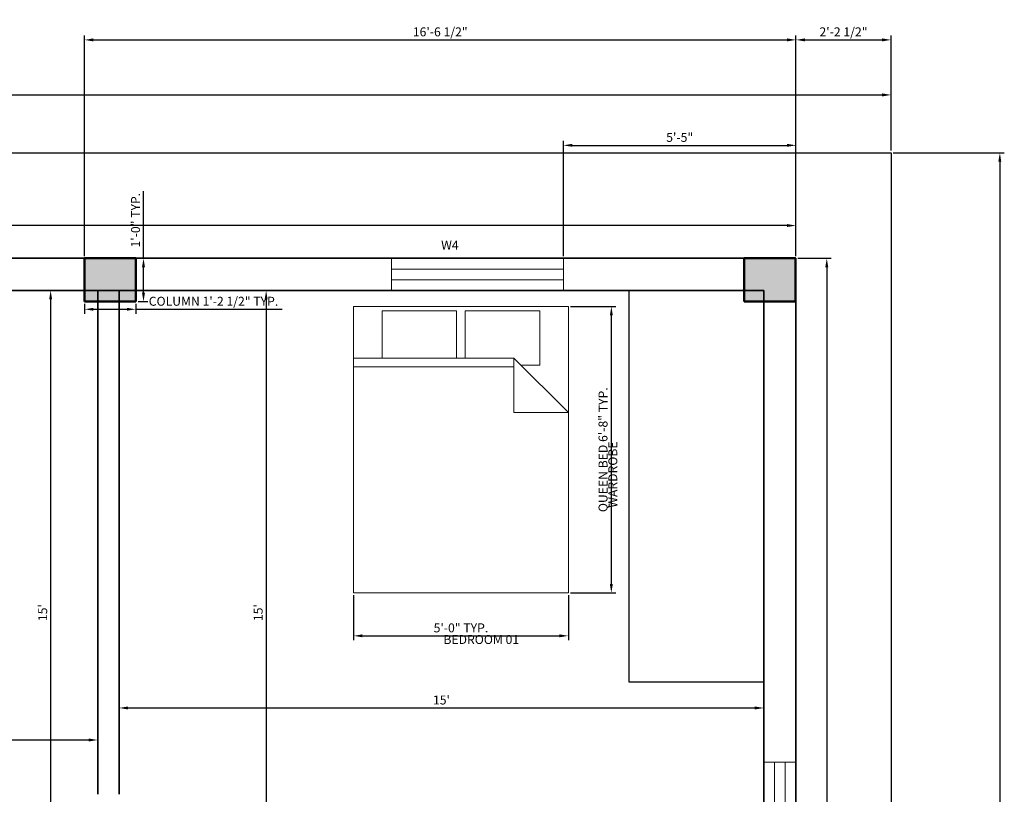
# Model space of a CAD drawing. Units: inches. Extents: x 2470 to 6338, y 1562 to 4199.
# Tile 4 of 5: x 2803 to 3078, y 1985 to 2201. Entities that reach past the tile are written whole.
import ezdxf

# ---------------------------------------------------------------- set-up
doc = ezdxf.new("R2010")
doc.units = ezdxf.units.IN
for name, color, linetype, lineweight in [('A-ANNO-DIMS', 2, 'Continuous', 18), ('A-ANNO-TEXT', 7, 'Continuous', 18), ('A-AREA-IDEN', 7, 'Continuous', 25), ('A-COLS', 1, 'Continuous', 50), ('A-FURN', 8, 'Continuous', 18), ('A-FURN-FIXD', 8, 'Continuous', 25), ('A-GLAZ', 4, 'Continuous', 18), ('A-WALL', 7, 'Continuous', 35), ('C-PROP', 3, 'Continuous', 25)]:
    doc.layers.add(name, color=color, linetype=linetype, lineweight=lineweight)
doc.styles.get("Standard").update_dxf_attribs({"font": 'arial.ttf'})
doc.dimstyles.new('ISO-25', dxfattribs={"dimtxt": 2.5, "dimasz": 2.5, "dimexe": 1.25, "dimexo": 0.625, "dimtad": 1, "dimdec": 1, "dimlunit": 3, "dimtxsty": 'Standard', "dimcen": 2.5, "dimadec": 0, "dimazin": 0, "dimtfac": 1, "dimtdec": 1, "dimtmove": 0, "dimatfit": 3, "dimfxl": 1, "dimarcsym": 0})

# ---------------------------------------------------------------- blocks, each defined once
blk = doc.blocks.new('Bed - Queen')
for p, q in [((0, -80.00003), (0, 0)), ((0, 0), (59.99999, 0)), ((59.99999, 0), (59.99999, -80.00003)), ((7.99999, -1.2), (28.79998, -1.2)), ((7.99999, -14.4), (7.99999, -1.2)), ((28.79998, -1.2), (28.79998, -14.4)), ((31.19999, -1.2), (51.99999, -1.2)), ((31.19999, -14.4), (31.19999, -1.2)), ((51.99999, -1.2), (51.99999, -16.4)), ((0, -14.4), (44.8, -14.4)), ((59.99999, -29.6), (44.8, -14.4)), ((44.8, -14.4), (44.8, -29.6)), ((51.99999, -16.4), (46.79936, -16.4)), ((44.8, -16.8), (0, -16.8)), ((44.8, -29.6), (59.99999, -29.6)), ((59.99999, -80.00003), (0, -80.00003))]:
    blk.add_line(p, q)
blk = doc.blocks.new('*D8')
at = {"layer": 'A-ANNO-DIMS', "color": 0, "lineweight": -2, "transparency": 16777216}
for p, q in [((2530.72, 2164.62), (2530.72, 2181.42)), ((3046.72, 2164.62), (3046.72, 2181.42)), ((2533.22, 2180.17), (3044.22, 2180.17))]:
    blk.add_line(p, q, dxfattribs=at)
at = {"layer": 'A-ANNO-DIMS', "color": 0, "lineweight": 100, "transparency": 16777216}
for points in [[(2533.22, 2180.59), (2533.22, 2179.75), (2530.72, 2180.17)], [(3044.22, 2180.59), (3044.22, 2179.75), (3046.72, 2180.17)]]:
    blk.add_solid(points, dxfattribs=at)
at = {"layer": 'Defpoints', "color": 0, "lineweight": 100, "transparency": 16777216}
for p in [(3046.72, 2180.17), (2530.72, 2163.99), (3046.72, 2163.99)]:
    blk.add_point(p, dxfattribs=at)
at = {"layer": 'A-ANNO-DIMS', "color": 0, "transparency": 16777216, "insert": (2788.72, 2182.07), "char_height": 2.5, "attachment_point": 5}
blk.add_mtext("43'", dxfattribs=at)
blk = doc.blocks.new('*D9')
at = {"layer": 'A-ANNO-DIMS', "color": 0, "lineweight": -2, "transparency": 16777216}
for p, q in [((3047.35, 2163.99), (3078.35, 2163.99)), ((3077.1, 2161.49), (3077.1, 1597.49)), ((3047.35, 1594.99), (3078.35, 1594.99))]:
    blk.add_line(p, q, dxfattribs=at)
at = {"layer": 'A-ANNO-DIMS', "color": 0, "lineweight": 100, "transparency": 16777216}
for points in [[(3076.68, 2161.49), (3077.51, 2161.49), (3077.1, 2163.99)], [(3076.68, 1597.49), (3077.51, 1597.49), (3077.1, 1594.99)]]:
    blk.add_solid(points, dxfattribs=at)
at = {"layer": 'Defpoints', "color": 0, "lineweight": 100, "transparency": 16777216}
for p in [(3046.72, 2163.99), (3046.72, 1594.99), (3077.1, 1594.99)]:
    blk.add_point(p, dxfattribs=at)
at = {"layer": 'A-ANNO-DIMS', "color": 0, "transparency": 16777216, "insert": (3075.2, 1879.49), "char_height": 2.5, "attachment_point": 5, "rotation": 90}
blk.add_mtext('47\'-5"', dxfattribs=at)
blk = doc.blocks.new('*D11')
at = {"layer": 'A-ANNO-DIMS', "color": 0, "lineweight": -2, "transparency": 16777216}
for p, q in [((2576.17, 2135.16), (2576.17, 2144.92)), ((3020.17, 2135.16), (3020.17, 2144.92)), ((3017.67, 2143.67), (2578.67, 2143.67))]:
    blk.add_line(p, q, dxfattribs=at)
at = {"layer": 'A-ANNO-DIMS', "color": 0, "lineweight": 100, "transparency": 16777216}
for points in [[(2578.67, 2144.09), (2578.67, 2143.26), (2576.17, 2143.67)], [(3017.67, 2144.09), (3017.67, 2143.26), (3020.17, 2143.67)]]:
    blk.add_solid(points, dxfattribs=at)
at = {"layer": 'Defpoints', "color": 0, "lineweight": 100, "transparency": 16777216}
for p in [(2576.17, 2143.67), (2576.17, 2134.53), (3020.17, 2134.53)]:
    blk.add_point(p, dxfattribs=at)
at = {"layer": 'A-ANNO-DIMS', "color": 0, "transparency": 16777216, "insert": (2798.17, 2145.58), "char_height": 2.5, "attachment_point": 5}
blk.add_mtext("37'", dxfattribs=at)
blk = doc.blocks.new('*D12')
at = {"layer": 'A-ANNO-DIMS', "color": 0, "lineweight": -2, "transparency": 16777216}
for p, q in [((3020.65, 2134.53), (3030.02, 2134.53)), ((3028.77, 2132.03), (3028.77, 1753.03)), ((3020.65, 1750.53), (3030.02, 1750.53))]:
    blk.add_line(p, q, dxfattribs=at)
at = {"layer": 'A-ANNO-DIMS', "color": 0, "lineweight": 100, "transparency": 16777216}
for points in [[(3028.36, 2132.03), (3029.19, 2132.03), (3028.77, 2134.53)], [(3028.36, 1753.03), (3029.19, 1753.03), (3028.77, 1750.53)]]:
    blk.add_solid(points, dxfattribs=at)
at = {"layer": 'Defpoints', "color": 0, "lineweight": 100, "transparency": 16777216}
for p in [(3020.03, 2134.53), (3020.03, 1750.53), (3028.77, 1750.53)]:
    blk.add_point(p, dxfattribs=at)
at = {"layer": 'A-ANNO-DIMS', "color": 0, "transparency": 16777216, "insert": (3026.87, 1942.53), "char_height": 2.5, "attachment_point": 5, "rotation": 90}
blk.add_mtext("32'", dxfattribs=at)
blk = doc.blocks.new('*D27')
at = {"layer": 'A-ANNO-DIMS', "color": 0, "lineweight": -2, "transparency": 16777216}
for p, q in [((2711.17, 2058.91), (2711.17, 1998.69)), ((2825.17, 2058.91), (2825.17, 1998.69)), ((2713.67, 1999.94), (2822.67, 1999.94))]:
    blk.add_line(p, q, dxfattribs=at)
at = {"layer": 'A-ANNO-DIMS', "color": 0, "lineweight": 100, "transparency": 16777216}
for points in [[(2713.67, 2000.36), (2713.67, 1999.53), (2711.17, 1999.94)], [(2822.67, 2000.36), (2822.67, 1999.53), (2825.17, 1999.94)]]:
    blk.add_solid(points, dxfattribs=at)
at = {"layer": 'Defpoints', "color": 0, "lineweight": 100, "transparency": 16777216}
for p in [(2711.17, 2059.53), (2825.17, 2059.53), (2825.17, 1999.94)]:
    blk.add_point(p, dxfattribs=at)
at = {"layer": 'A-ANNO-DIMS', "color": 0, "transparency": 16777216, "insert": (2768.17, 2001.84), "char_height": 2.5, "attachment_point": 5}
blk.add_mtext('9\'-6"', dxfattribs=at)
blk = doc.blocks.new('*D28')
at = {"layer": 'A-ANNO-DIMS', "color": 0, "lineweight": -2, "transparency": 16777216}
for p, q in [((2808.15, 2125.53), (2813.28, 2125.53)), ((2812.03, 2123.03), (2812.03, 1948.03)), ((2808.15, 1945.53), (2813.28, 1945.53))]:
    blk.add_line(p, q, dxfattribs=at)
at = {"layer": 'A-ANNO-DIMS', "color": 0, "lineweight": 100, "transparency": 16777216}
for points in [[(2811.62, 2123.03), (2812.45, 2123.03), (2812.03, 2125.53)], [(2811.62, 1948.03), (2812.45, 1948.03), (2812.03, 1945.53)]]:
    blk.add_solid(points, dxfattribs=at)
at = {"layer": 'Defpoints', "color": 0, "lineweight": 100, "transparency": 16777216}
for p in [(2807.53, 2125.53), (2807.53, 1945.53), (2812.03, 1945.53)]:
    blk.add_point(p, dxfattribs=at)
at = {"layer": 'A-ANNO-DIMS', "color": 0, "transparency": 16777216, "insert": (2810.13, 2035.53), "char_height": 2.5, "attachment_point": 5, "rotation": 90}
blk.add_mtext("15'", dxfattribs=at)
blk = doc.blocks.new('*D29')
at = {"layer": 'A-ANNO-DIMS', "color": 0, "lineweight": -2, "transparency": 16777216}
for p, q in [((2831.17, 2010.54), (2831.17, 2007.64)), ((3011.17, 2010.54), (3011.17, 2007.64)), ((2833.67, 2008.89), (3008.67, 2008.89))]:
    blk.add_line(p, q, dxfattribs=at)
at = {"layer": 'A-ANNO-DIMS', "color": 0, "lineweight": 100, "transparency": 16777216}
for points in [[(2833.67, 2009.31), (2833.67, 2008.47), (2831.17, 2008.89)], [(3008.67, 2009.31), (3008.67, 2008.47), (3011.17, 2008.89)]]:
    blk.add_solid(points, dxfattribs=at)
at = {"layer": 'Defpoints', "color": 0, "lineweight": 100, "transparency": 16777216}
for p in [(2831.17, 2011.17), (3011.17, 2011.17), (3011.17, 2008.89)]:
    blk.add_point(p, dxfattribs=at)
at = {"layer": 'A-ANNO-DIMS', "color": 0, "transparency": 16777216, "insert": (2921.17, 2010.79), "char_height": 2.5, "attachment_point": 5}
blk.add_mtext("15'", dxfattribs=at)
blk = doc.blocks.new('*D30')
at = {"layer": 'A-ANNO-DIMS', "color": 0, "lineweight": -2, "transparency": 16777216}
for p, q in [((2859.5, 2125.53), (2873.46, 2125.53)), ((2872.21, 2123.03), (2872.21, 1948.03)), ((2867.05, 1945.53), (2873.46, 1945.53))]:
    blk.add_line(p, q, dxfattribs=at)
at = {"layer": 'A-ANNO-DIMS', "color": 0, "lineweight": 100, "transparency": 16777216}
for points in [[(2871.79, 2123.03), (2872.62, 2123.03), (2872.21, 2125.53)], [(2871.79, 1948.03), (2872.62, 1948.03), (2872.21, 1945.53)]]:
    blk.add_solid(points, dxfattribs=at)
at = {"layer": 'Defpoints', "color": 0, "lineweight": 100, "transparency": 16777216}
for p in [(2858.88, 2125.53), (2866.42, 1945.53), (2872.21, 1945.53)]:
    blk.add_point(p, dxfattribs=at)
at = {"layer": 'A-ANNO-DIMS', "color": 0, "transparency": 16777216, "insert": (2870.31, 2035.53), "char_height": 2.5, "attachment_point": 5, "rotation": 90}
blk.add_mtext("15'", dxfattribs=at)
blk = doc.blocks.new('WIN-48IN')
for p, q in [((0, 9), (48, 9)), ((0, 0), (0, 9)), ((48, 9), (48, 0)), ((0, 6), (48, 6)), ((48, 3), (0, 3)), ((48, 0), (0, 0))]:
    blk.add_line(p, q)
blk = doc.blocks.new('COL-RECT-LARGE')
h = blk.add_hatch(color=256)
h.dxf.hatch_style = 1
h.paths.add_polyline_path([(14.33, 12.11), (10, 12.11), (0, 12.11), (0, 0), (10, 0), (14.33, 0)])
for p, q in [((10, 12.11), (0, 12.11)), ((0, 12.11), (0, 0)), ((10, 12.11), (14.33, 12.11)), ((14.33, 12.11), (14.33, 0)), ((10, 0), (0, 0)), ((14.33, 0), (10, 0))]:
    blk.add_line(p, q)
blk = doc.blocks.new('*D40')
at = {"layer": 'A-ANNO-DIMS', "color": 0, "lineweight": -2, "transparency": 16777216}
for p, q in [((2821.49, 2121.8), (2821.49, 2119.03)), ((2823.99, 2120.28), (2833.31, 2120.28)), ((2835.81, 2121.8), (2835.81, 2119.03)), ((2835.81, 2120.28), (2876.7, 2120.28))]:
    blk.add_line(p, q, dxfattribs=at)
at = {"layer": 'A-ANNO-DIMS', "color": 0, "lineweight": 100, "transparency": 16777216}
for points in [[(2823.99, 2120.69), (2823.99, 2119.86), (2821.49, 2120.28)], [(2833.31, 2120.69), (2833.31, 2119.86), (2835.81, 2120.28)]]:
    blk.add_solid(points, dxfattribs=at)
at = {"layer": 'Defpoints', "color": 0, "lineweight": 100, "transparency": 16777216}
for p in [(2821.49, 2122.42), (2835.81, 2122.42), (2835.81, 2120.28)]:
    blk.add_point(p, dxfattribs=at)
at = {"layer": 'A-ANNO-DIMS', "color": 0, "transparency": 16777216, "insert": (2857.51, 2122.19), "char_height": 2.5, "attachment_point": 5}
blk.add_mtext('COLUMN 1\'-2 1/2" TYP.', dxfattribs=at)
blk = doc.blocks.new('*D41')
at = {"layer": 'A-ANNO-DIMS', "color": 0, "lineweight": -2, "transparency": 16777216}
for p, q in [((2837.96, 2134.53), (2837.96, 2153.29)), ((2836.44, 2134.53), (2839.21, 2134.53)), ((2837.96, 2124.92), (2837.96, 2132.03)), ((2836.44, 2122.42), (2839.21, 2122.42))]:
    blk.add_line(p, q, dxfattribs=at)
at = {"layer": 'A-ANNO-DIMS', "color": 0, "lineweight": 100, "transparency": 16777216}
for points in [[(2837.54, 2132.03), (2838.38, 2132.03), (2837.96, 2134.53)], [(2837.54, 2124.92), (2838.38, 2124.92), (2837.96, 2122.42)]]:
    blk.add_solid(points, dxfattribs=at)
at = {"layer": 'Defpoints', "color": 0, "lineweight": 100, "transparency": 16777216}
for p in [(2835.81, 2134.53), (2837.96, 2134.53), (2835.81, 2122.42)]:
    blk.add_point(p, dxfattribs=at)
at = {"layer": 'A-ANNO-DIMS', "color": 0, "transparency": 16777216, "insert": (2836.06, 2145.16), "char_height": 2.5, "attachment_point": 5, "rotation": 90}
blk.add_mtext('1\'-0" TYP.', dxfattribs=at)
blk = doc.blocks.new('*D46')
at = {"layer": 'A-ANNO-DIMS', "color": 0, "lineweight": -2, "transparency": 16777216}
for p, q in [((2957.23, 2121.04), (2969.86, 2121.04)), ((2968.61, 2043.54), (2968.61, 2118.54)), ((2957.23, 2041.04), (2969.86, 2041.04))]:
    blk.add_line(p, q, dxfattribs=at)
at = {"layer": 'A-ANNO-DIMS', "color": 0, "lineweight": 100, "transparency": 16777216}
for points in [[(2968.19, 2118.54), (2969.03, 2118.54), (2968.61, 2121.04)], [(2968.19, 2043.54), (2969.03, 2043.54), (2968.61, 2041.04)]]:
    blk.add_solid(points, dxfattribs=at)
at = {"layer": 'Defpoints', "color": 0, "lineweight": 100, "transparency": 16777216}
for p in [(2956.61, 2121.04), (2968.61, 2121.04), (2956.61, 2041.04)]:
    blk.add_point(p, dxfattribs=at)
at = {"layer": 'A-ANNO-DIMS', "color": 0, "transparency": 16777216, "insert": (2966.61, 2081.04), "char_height": 2.5, "attachment_point": 5, "rotation": 90}
blk.add_mtext('QUEEN BED 6\'-8" TYP.', dxfattribs=at)
blk = doc.blocks.new('*D47')
at = {"layer": 'A-ANNO-DIMS', "color": 0, "lineweight": -2, "transparency": 16777216}
for p, q in [((2896.61, 2040.42), (2896.61, 2027.79)), ((2956.61, 2040.42), (2956.61, 2027.79)), ((2899.11, 2029.04), (2954.11, 2029.04))]:
    blk.add_line(p, q, dxfattribs=at)
at = {"layer": 'A-ANNO-DIMS', "color": 0, "lineweight": 100, "transparency": 16777216}
for points in [[(2899.11, 2029.46), (2899.11, 2028.63), (2896.61, 2029.04)], [(2954.11, 2029.46), (2954.11, 2028.63), (2956.61, 2029.04)]]:
    blk.add_solid(points, dxfattribs=at)
at = {"layer": 'Defpoints', "color": 0, "lineweight": 100, "transparency": 16777216}
for p in [(2896.61, 2041.04), (2956.61, 2041.04), (2956.61, 2029.04)]:
    blk.add_point(p, dxfattribs=at)
at = {"layer": 'A-ANNO-DIMS', "color": 0, "transparency": 16777216, "insert": (2926.61, 2030.94), "char_height": 2.5, "attachment_point": 5}
blk.add_mtext('5\'-0" TYP.', dxfattribs=at)
blk = doc.blocks.new('*D61')
at = {"layer": 'A-ANNO-DIMS', "color": 0, "lineweight": -2, "transparency": 16777216}
for p, q in [((2821.49, 2135.16), (2821.49, 2196.79)), ((2823.99, 2195.54), (3017.67, 2195.54)), ((3020.17, 2135.16), (3020.17, 2196.79))]:
    blk.add_line(p, q, dxfattribs=at)
at = {"layer": 'A-ANNO-DIMS', "color": 0, "lineweight": 100, "transparency": 16777216}
for points in [[(2823.99, 2195.96), (2823.99, 2195.12), (2821.49, 2195.54)], [(3017.67, 2195.96), (3017.67, 2195.12), (3020.17, 2195.54)]]:
    blk.add_solid(points, dxfattribs=at)
at = {"layer": 'Defpoints', "color": 0, "lineweight": 100, "transparency": 16777216}
for p in [(3020.17, 2195.54), (2821.49, 2134.53), (3020.17, 2134.53)]:
    blk.add_point(p, dxfattribs=at)
at = {"layer": 'A-ANNO-DIMS', "color": 0, "transparency": 16777216, "insert": (2920.83, 2197.46), "char_height": 2.5, "attachment_point": 5}
blk.add_mtext('16\'-6 1/2"', dxfattribs=at)
blk = doc.blocks.new('*D66')
at = {"layer": 'A-ANNO-DIMS', "color": 0, "lineweight": -2, "transparency": 16777216}
for p, q in [((3020.17, 2135.16), (3020.17, 2196.79)), ((3022.67, 2195.54), (3044.22, 2195.54)), ((3046.72, 2164.62), (3046.72, 2196.79))]:
    blk.add_line(p, q, dxfattribs=at)
at = {"layer": 'A-ANNO-DIMS', "color": 0, "lineweight": 100, "transparency": 16777216}
for points in [[(3022.67, 2195.96), (3022.67, 2195.12), (3020.17, 2195.54)], [(3044.22, 2195.96), (3044.22, 2195.12), (3046.72, 2195.54)]]:
    blk.add_solid(points, dxfattribs=at)
at = {"layer": 'Defpoints', "color": 0, "lineweight": 100, "transparency": 16777216}
for p in [(3046.72, 2195.54), (3046.72, 2163.99), (3020.17, 2134.53)]:
    blk.add_point(p, dxfattribs=at)
at = {"layer": 'A-ANNO-DIMS', "color": 0, "transparency": 16777216, "insert": (3033.44, 2197.46), "char_height": 2.5, "attachment_point": 5}
blk.add_mtext('2\'-2 1/2"', dxfattribs=at)
blk = doc.blocks.new('*D72')
at = {"layer": 'A-ANNO-DIMS', "color": 0, "lineweight": -2, "transparency": 16777216}
for p, q in [((2955.23, 2135.16), (2955.23, 2167.33)), ((3020.17, 2135.16), (3020.17, 2167.33)), ((2957.73, 2166.08), (3017.67, 2166.08))]:
    blk.add_line(p, q, dxfattribs=at)
at = {"layer": 'A-ANNO-DIMS', "color": 0, "lineweight": 100, "transparency": 16777216}
for points in [[(2957.73, 2166.5), (2957.73, 2165.67), (2955.23, 2166.08)], [(3017.67, 2166.5), (3017.67, 2165.67), (3020.17, 2166.08)]]:
    blk.add_solid(points, dxfattribs=at)
at = {"layer": 'Defpoints', "color": 0, "lineweight": 100, "transparency": 16777216}
for p in [(3020.17, 2166.08), (2955.23, 2134.53), (3020.17, 2134.53)]:
    blk.add_point(p, dxfattribs=at)
at = {"layer": 'A-ANNO-DIMS', "color": 0, "transparency": 16777216, "insert": (2987.7, 2167.98), "char_height": 2.5, "attachment_point": 5}
blk.add_mtext('5\'-5"', dxfattribs=at)

msp = doc.modelspace()

# ---------------------------------------------------------------- linework, layer by layer
at = {"layer": 'A-FURN-FIXD'}
for p, q in [((2973.48, 2125.53), (2973.48, 2016.18)), ((2973.48, 2016.18), (3011.17, 2016.18))]:
    msp.add_line(p, q, dxfattribs=at)
at = {"layer": 'A-WALL'}
for p, q in [((2576.17, 2134.53), (3020.17, 2134.53)), ((3020.17, 2134.53), (3020.17, 1750.53)), ((2585.17, 2125.53), (3011.17, 2125.53)), ((2825.17, 2125.53), (2825.17, 1984.76)), ((2831.17, 2125.53), (2831.17, 1984.76)), ((3011.17, 2125.53), (3011.17, 1852.53))]:
    msp.add_line(p, q, dxfattribs=at)
at = {"layer": 'C-PROP'}
for p, q in [((2530.72, 2163.99), (3046.72, 2163.99)), ((3046.72, 2163.99), (3046.72, 1594.99))]:
    msp.add_line(p, q, dxfattribs=at)

# ---------------------------------------------------------------- block references
at = {"layer": 'A-COLS'}
for p in [(2821.49, 2122.42), (3005.7, 2122.42)]:
    msp.add_blockref('COL-RECT-LARGE', p, dxfattribs=at)
at = {"layer": 'A-FURN'}
msp.add_blockref('Bed - Queen', (2896.61, 2121.04), dxfattribs=at)
at = {"layer": 'A-GLAZ'}
msp.add_blockref('WIN-48IN', (2907.23, 2125.53), dxfattribs=at)
at = {"layer": 'A-GLAZ', "rotation": 89.9999999999996}
msp.add_blockref('WIN-48IN', (3020.17, 1945.73), dxfattribs=at)

# ---------------------------------------------------------------- texts
at = {"layer": 'A-ANNO-TEXT', "insert": (2921.08, 2139.44), "char_height": 2.5, "attachment_point": 1}
msp.add_mtext_dynamic_manual_height_columns('W4', width=14.944, gutter_width=12.5, heights=[0], dxfattribs=at)
at = {"layer": 'A-ANNO-TEXT', "insert": (2967.77, 2064.83), "char_height": 2.5, "attachment_point": 1, "rotation": 90}
msp.add_mtext_dynamic_manual_height_columns('WARDROBE', width=31.0449, gutter_width=12.5, heights=[0], dxfattribs=at)
at = {"layer": 'A-AREA-IDEN', "insert": (2921.71, 2029.26), "char_height": 2.5, "attachment_point": 1}
msp.add_mtext_dynamic_manual_height_columns('BEDROOM 01', width=53.323, gutter_width=12.5, heights=[0], dxfattribs=at)

# ---------------------------------------------------------------- dimensions: what is measured, and where the dimension line sits
at = {"layer": 'A-ANNO-DIMS'}
for base, p1, p2, override, picture, middle in [((3020.17, 2195.54), (2821.49, 2134.53), (3020.17, 2134.53), {"dimdec": 1, "dimlfac": 1, "dimrnd": 0, "dimzin": 1, "dimdsep": 46, "dimlunit": 4, "dimfrac": 2}, '*D61', (2920.83, 2197.46)), ((3046.7223, 2195.5407), (3020.1674, 2134.5342), (3046.7223, 2163.9907), {"dimdec": 1, "dimlfac": 1, "dimrnd": 0, "dimzin": 1, "dimdsep": 46, "dimlunit": 4, "dimfrac": 2}, '*D66', (3033.4449, 2197.4584)), ((3046.72, 2180.17), (2530.72, 2163.99), (3046.72, 2163.99), {"dimclrd": 0, "dimclre": 0, "dimclrt": 0}, '*D8', (2788.72, 2182.07)), ((3020.17, 2166.08), (2955.23, 2134.53), (3020.17, 2134.53), {"dimdec": 1, "dimlfac": 1, "dimrnd": 0, "dimzin": 1, "dimdsep": 46, "dimlunit": 4, "dimfrac": 2}, '*D72', (2987.7, 2167.98)), ((2576.17, 2143.67), (3020.17, 2134.53), (2576.17, 2134.53), {"dimclrd": 0, "dimclre": 0, "dimclrt": 0}, '*D11', (2798.17, 2145.58)), ((2825.17, 1999.94), (2711.17, 2059.53), (2825.17, 2059.53), {"dimclrd": 0, "dimclre": 0, "dimclrt": 0}, '*D27', (2768.17, 2001.84)), ((3011.17, 2008.89), (2831.17, 2011.17), (3011.17, 2011.17), {"dimclrd": 0, "dimclre": 0, "dimclrt": 0}, '*D29', (2921.17, 2010.79))]:
    dim = msp.add_linear_dim(base=base, p1=p1, p2=p2, dimstyle='ISO-25', override=override, dxfattribs=at)
    dim.commit()
    dim.dimension.update_dxf_attribs({"geometry": picture, "text_midpoint": middle})
for base, p1, p2, picture, middle in [((3077.1, 1594.99), (3046.72, 2163.99), (3046.72, 1594.99), '*D9', (3075.2, 1879.49)), ((3028.77, 1750.53), (3020.03, 2134.53), (3020.03, 1750.53), '*D12', (3026.87, 1942.53)), ((2812.03, 1945.53), (2807.53, 2125.53), (2807.53, 1945.53), '*D28', (2810.13, 2035.53)), ((2872.21, 1945.53), (2858.88, 2125.53), (2866.42, 1945.53), '*D30', (2870.31, 2035.53))]:
    dim = msp.add_linear_dim(base=base, p1=p1, p2=p2, angle=90, dimstyle='ISO-25', override={"dimclrd": 0, "dimclre": 0, "dimclrt": 0}, dxfattribs=at)
    dim.commit()
    dim.dimension.update_dxf_attribs({"geometry": picture, "text_midpoint": middle})
for base, p1, p2, text, picture, middle in [((2837.96, 2134.53), (2835.81, 2122.42), (2835.81, 2134.53), '<> TYP.', '*D41', (2836.06, 2145.16)), ((2968.61, 2121.04), (2956.61, 2041.04), (2956.61, 2121.04), 'QUEEN BED <> TYP.', '*D46', (2966.61, 2081.04))]:
    dim = msp.add_linear_dim(base=base, p1=p1, p2=p2, angle=90, text=text, dimstyle='ISO-25', override={"dimdec": 1, "dimlfac": 1, "dimrnd": 0, "dimzin": 1, "dimdsep": 46, "dimlunit": 4, "dimfrac": 2}, dxfattribs=at)
    dim.commit()
    dim.dimension.update_dxf_attribs({"geometry": picture, "text_midpoint": middle})
for base, p1, p2, text, picture, middle in [((2835.81, 2120.28), (2821.49, 2122.42), (2835.81, 2122.42), 'COLUMN <> TYP.', '*D40', (2857.51, 2122.19)), ((2956.61, 2029.04), (2896.61, 2041.04), (2956.61, 2041.04), '<> TYP.', '*D47', (2926.61, 2030.94))]:
    dim = msp.add_linear_dim(base=base, p1=p1, p2=p2, text=text, dimstyle='ISO-25', override={"dimdec": 1, "dimlfac": 1, "dimrnd": 0, "dimzin": 1, "dimdsep": 46, "dimlunit": 4, "dimfrac": 2}, dxfattribs=at)
    dim.commit()
    dim.dimension.update_dxf_attribs({"geometry": picture, "text_midpoint": middle})

doc.saveas('drawing.dxf')
